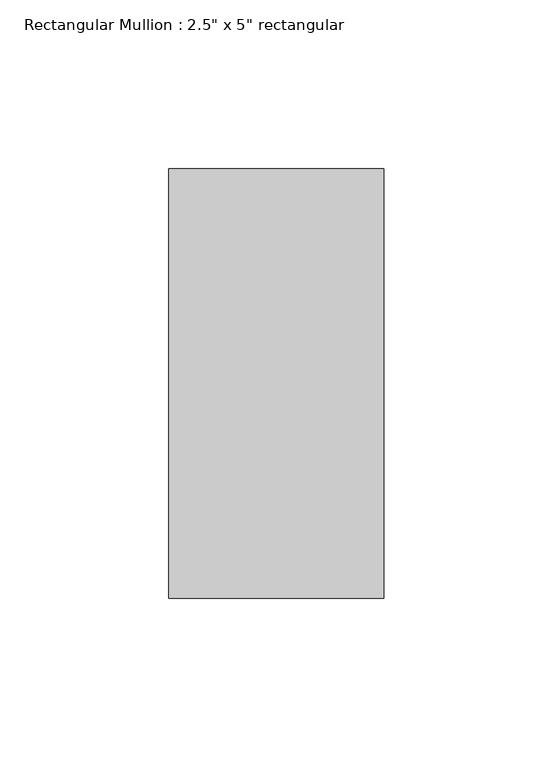
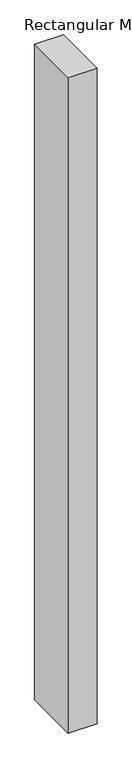
"""IFC4 building model written with IfcOpenShell, lengths in millimetres: member geometry."""

from ifc_helpers import new_model, si_unit, frame, origin, place, context, project, spatial, polyline, outline, extrude, source, transform, mapped, element, save


def member_4491d118(model_context):
    return source(origin(), model_context, "Body", "SweptSolid", [
        extrude(outline(polyline([(0.0, 63.5), (0.0, -63.5), (-63.5, -63.5), (-63.5, 63.5), (0.0, 63.5)])), frame((0.0, 0.0, -1524.0), z_axis=(0.0, 0.0, 1.0), x_axis=(1.0, 0.0, 0.0)), (0.0, 0.0, 1.0), 1524.0),
    ])


if __name__ == "__main__":
    model = new_model("IFC4")
    model_context = context("Model", 3, world=origin())
    ifc_project = project(units=[si_unit("LENGTHUNIT", "METRE", prefix="MILLI")], contexts=[model_context])
    site = spatial("IfcSite", under=ifc_project)
    building = spatial("IfcBuilding", under=site)
    placement = place(None, origin())
    member_shape = member_4491d118(model_context)
    element("IfcMember", 1, ObjectType="Rectangular Mullion : 2.5\" x 5\" rectangular", at=placement, inside=building, context=model_context, shape_type="MappedRepresentation", body=[
        mapped(member_shape, transform((0.0, 0.0, 0.0), x_axis=(1.0, 0.0, 0.0), y_axis=(0.0, 1.0, 0.0), z_axis=(0.0, 0.0, 1.0))),
    ])
    save(model, "model.ifc")

# Revit data of these elements
# Type "Rectangular Mullion : 2.5\" x 5\" rectangular"
#   built-in parameter 1007304 = 0.416667 (stored number, unit not read)
#   built-in parameter 1007301 = 0.104167 (stored number, unit not read)
#   built-in parameter 1007300 = 0.104167 (stored number, unit not read)
